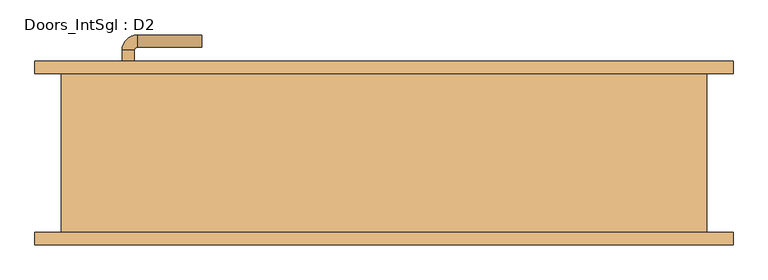
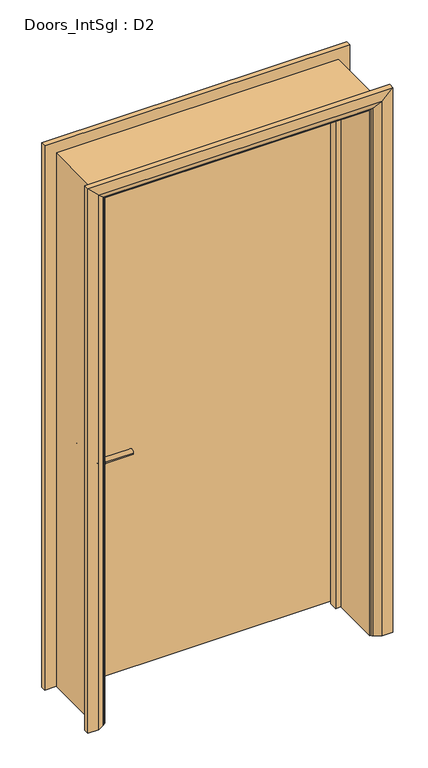
"""IFC4 building model written with IfcOpenShell, lengths in millimetres: door geometry, Doors_IntSgl : D2."""

from ifc_helpers import new_model, si_unit, point, frame, frame_2d, origin, place, context, project, spatial, polyline, circle_curve, ellipse_curve, trimmed, segment, composite_curve, outline, extrude, faceted_brep, source, transform, mapped, element, save
from ifc_brep_helpers import plane_surface, cylinder_surface, revolved_surface, advanced_brep


def doors_intsgl_d2_0f955423(model_context):
    return source(origin(), model_context, "Body", "SolidModel", [
        advanced_brep(
        [(-426.4, 83.54, 900.0), (-406.4, 83.54, 900.0), (-406.4, 53.54, 900.0), (-426.4, 53.54, 900.0), (-401.4, 48.54, 900.0), (-401.4, 28.54, 900.0), (-296.4, 28.54, 900.0), (-296.4, 48.54, 900.0)],
        [
            (0, 1, circle_curve(frame((-416.4, 83.54, 900.0), z_axis=(0.0, 1.0, 0.0), x_axis=(1.0, 0.0, 0.0)), 10.0)),
            (1, 0, circle_curve(frame((-416.4, 83.54, 900.0), z_axis=(0.0, 1.0, 0.0), x_axis=(1.0, 0.0, 0.0)), 10.0)),
            (1, 2),
            (2, 3, circle_curve(frame((-416.4, 53.54, 900.0), z_axis=(0.0, 1.0, 0.0), x_axis=(1.0, 0.0, 0.0)), 10.0)),
            (3, 0),
            (3, 2, circle_curve(frame((-416.4, 53.54, 900.0), z_axis=(0.0, 1.0, 0.0), x_axis=(1.0, 0.0, 0.0)), 10.0)),
            (4, 5, circle_curve(frame((-401.4, 38.54, 900.0), z_axis=(-1.0, 0.0, 0.0), x_axis=(0.0, 1.0, 0.0)), 10.0)),
            (5, 3, circle_curve(frame((-401.4, 53.54, 900.0), z_axis=(0.0, 0.0, -1.0), x_axis=(-1.0, 0.0, 0.0)), 25.0)),
            (2, 4, circle_curve(frame((-401.4, 53.54, 900.0), z_axis=(0.0, 0.0, 1.0), x_axis=(-1.0, 0.0, 0.0)), 5.0)),
            (5, 4, circle_curve(frame((-401.4, 38.54, 900.0), z_axis=(-1.0, 0.0, 0.0), x_axis=(0.0, 1.0, 0.0)), 10.0)),
            (6, 7, circle_curve(frame((-296.4, 38.54, 900.0), z_axis=(1.0, 0.0, 0.0), x_axis=(0.0, 1.0, 0.0)), 10.0)),
            (7, 6, circle_curve(frame((-296.4, 38.54, 900.0), z_axis=(1.0, 0.0, 0.0), x_axis=(0.0, 1.0, 0.0)), 10.0)),
            (4, 7),
            (6, 5),
        ],
        [
            plane_surface(frame((-416.4, 83.54, 900.0), z_axis=(0.0, 1.0, 0.0), x_axis=(0.0, 0.0, 1.0))),
            cylinder_surface(frame((-416.4, 83.54, 900.0), z_axis=(0.0, 1.0, 0.0), x_axis=(1.0, 0.0, 0.0)), 10.0),
            revolved_surface(trimmed(ellipse_curve(frame((-416.4, 53.54, 900.0), z_axis=(0.0, -1.0, 0.0), x_axis=(1.0, 0.0, 0.0)), 10.0, 10.0), [point((-426.4, 53.54, 900.0))], [point((-406.4, 53.54, 900.0))], True, "CARTESIAN"), (-401.4, 53.54, 900.0), (0.0, 0.0, -1.0)),
            revolved_surface(trimmed(ellipse_curve(frame((-416.4, 53.54, 900.0), z_axis=(0.0, -1.0, 0.0), x_axis=(1.0, 0.0, 0.0)), 10.0, 10.0), [point((-406.4, 53.54, 900.0))], [point((-426.4, 53.54, 900.0))], True, "CARTESIAN"), (-401.4, 53.54, 900.0), (0.0, 0.0, -1.0)),
            plane_surface(frame((-296.4, 38.54, 900.0), z_axis=(1.0, 0.0, 0.0), x_axis=(0.0, 0.0, 1.0))),
            cylinder_surface(frame((-401.4, 38.54, 900.0), z_axis=(-1.0, 0.0, 0.0), x_axis=(0.0, 1.0, 0.0)), 10.0),
        ],
        [
            (0, [[1, 2]]),
            (1, [[3, 4, 5, -2]]),
            (1, [[-5, 6, -3, -1]]),
            (2, [[7, 8, -4, 9]]),
            (3, [[10, -9, -6, -8]]),
            (4, [[11, 12]]),
            (5, [[13, -11, 14, -7]]),
            (5, [[-14, -12, -13, -10]]),
        ],
    ),
        extrude(outline(composite_curve([segment(trimmed(circle_curve(frame_2d((900.0, -418.9)), 30.0), [point((900.0, -448.9))], [point((900.0, -388.9))], False, "CARTESIAN"), True, "CONTINUOUS"), segment(trimmed(circle_curve(frame_2d((900.0, -418.9)), 30.0), [point((900.0, -388.9))], [point((900.0, -448.9))], False, "CARTESIAN"), True, "CONTINUOUS")], self_intersect=False)), frame((0.0, 83.54, 0.0), z_axis=(0.0, 1.0, 0.0), x_axis=(0.0, 0.0, 1.0)), (0.0, 0.0, 1.0), 8.0),
        advanced_brep(
        [(-426.4, 137.54, 900.0), (-406.4, 137.54, 900.0), (-426.4, 167.54, 900.0), (-406.4, 167.54, 900.0), (-401.4, 172.54, 900.0), (-401.4, 192.54, 900.0), (-296.4, 192.54, 900.0), (-296.4, 172.54, 900.0)],
        [
            (0, 1, circle_curve(frame((-416.4, 137.54, 900.0), z_axis=(0.0, -1.0, 0.0), x_axis=(1.0, 0.0, 0.0)), 10.0)),
            (1, 0, circle_curve(frame((-416.4, 137.54, 900.0), z_axis=(0.0, -1.0, 0.0), x_axis=(1.0, 0.0, 0.0)), 10.0)),
            (0, 2),
            (2, 3, circle_curve(frame((-416.4, 167.54, 900.0), z_axis=(0.0, -1.0, 0.0), x_axis=(1.0, 0.0, 0.0)), 10.0)),
            (3, 1),
            (3, 2, circle_curve(frame((-416.4, 167.54, 900.0), z_axis=(0.0, -1.0, 0.0), x_axis=(1.0, 0.0, 0.0)), 10.0)),
            (4, 3, circle_curve(frame((-401.4, 167.54, 900.0), z_axis=(0.0, 0.0, 1.0), x_axis=(-1.0, 0.0, 0.0)), 5.0)),
            (2, 5, circle_curve(frame((-401.4, 167.54, 900.0), z_axis=(0.0, 0.0, -1.0), x_axis=(-1.0, 0.0, 0.0)), 25.0)),
            (5, 4, circle_curve(frame((-401.4, 182.54, 900.0), z_axis=(-1.0, 0.0, 0.0), x_axis=(0.0, -1.0, 0.0)), 10.0)),
            (4, 5, circle_curve(frame((-401.4, 182.54, 900.0), z_axis=(-1.0, 0.0, 0.0), x_axis=(0.0, -1.0, 0.0)), 10.0)),
            (6, 7, circle_curve(frame((-296.4, 182.54, 900.0), z_axis=(1.0, 0.0, 0.0), x_axis=(0.0, -1.0, 0.0)), 10.0)),
            (7, 6, circle_curve(frame((-296.4, 182.54, 900.0), z_axis=(1.0, 0.0, 0.0), x_axis=(0.0, -1.0, 0.0)), 10.0)),
            (5, 6),
            (7, 4),
        ],
        [
            plane_surface(frame((-416.4, 137.54, 900.0), z_axis=(0.0, -1.0, 0.0), x_axis=(0.0, 0.0, 1.0))),
            cylinder_surface(frame((-416.4, 137.54, 900.0), z_axis=(0.0, -1.0, 0.0), x_axis=(1.0, 0.0, 0.0)), 10.0),
            revolved_surface(trimmed(ellipse_curve(frame((-416.4, 167.54, 900.0), z_axis=(0.0, -1.0, 0.0), x_axis=(1.0, 0.0, 0.0)), 10.0, 10.0), [point((-426.4, 167.54, 900.0))], [point((-406.4, 167.54, 900.0))], True, "CARTESIAN"), (-401.4, 167.54, 900.0), (0.0, 0.0, -1.0)),
            revolved_surface(trimmed(ellipse_curve(frame((-416.4, 167.54, 900.0), z_axis=(0.0, -1.0, 0.0), x_axis=(1.0, 0.0, 0.0)), 10.0, 10.0), [point((-406.4, 167.54, 900.0))], [point((-426.4, 167.54, 900.0))], True, "CARTESIAN"), (-401.4, 167.54, 900.0), (0.0, 0.0, -1.0)),
            plane_surface(frame((-296.4, 182.54, 900.0), z_axis=(1.0, 0.0, 0.0), x_axis=(0.0, 0.0, 1.0))),
            cylinder_surface(frame((-401.4, 182.54, 900.0), z_axis=(-1.0, 0.0, 0.0), x_axis=(0.0, -1.0, 0.0)), 10.0),
        ],
        [
            (0, [[1, 2]]),
            (1, [[-1, 3, 4, 5]]),
            (1, [[-2, -5, 6, -3]]),
            (2, [[7, -4, 8, 9]]),
            (3, [[-8, -6, -7, 10]]),
            (4, [[11, 12]]),
            (5, [[-9, 13, -12, 14]]),
            (5, [[-10, -14, -11, -13]]),
        ],
    ),
        extrude(outline(composite_curve([segment(trimmed(circle_curve(frame_2d((900.0, -418.9)), 30.0), [point((900.0, -448.9))], [point((900.0, -388.9))], False, "CARTESIAN"), True, "CONTINUOUS"), segment(trimmed(circle_curve(frame_2d((900.0, -418.9)), 30.0), [point((900.0, -388.9))], [point((900.0, -448.9))], False, "CARTESIAN"), True, "CONTINUOUS")], self_intersect=False)), frame((0.0, 129.54, 0.0), z_axis=(0.0, 1.0, 0.0), x_axis=(0.0, 0.0, 1.0)), (0.0, 0.0, 1.0), 8.0),
        extrude(outline(polyline([(491.4, 91.54), (-491.4, 91.54), (-491.4, 129.54), (491.4, 129.54), (491.4, 91.54)])), frame((0.0, 0.0, 8.0), z_axis=(0.0, 0.0, 1.0), x_axis=(1.0, 0.0, 0.0)), (0.0, 0.0, 1.0), 2060.0),
        advanced_brep(
        [(568.4, 149.54, 0.0), (568.4, 129.54, 0.0), (498.4, 129.54, 0.0), (502.4, 135.54, 0.0), (528.4, 149.54, 0.0), (568.4, 149.54, 2145.0), (568.4, 129.54, 2145.0), (-568.4, 129.54, 2145.0), (-568.4, 129.54, 0.0), (-498.4, 129.54, 0.0), (-498.4, 129.54, 2075.0), (498.4, 129.54, 2075.0), (502.4, 135.54, 2079.0), (528.4, 149.54, 2105.0), (-528.4, 149.54, 2105.0), (-528.4, 149.54, 0.0), (-568.4, 149.54, 0.0), (-568.4, 149.54, 2145.0), (-502.4, 135.54, 0.0), (-502.4, 135.54, 2079.0)],
        [
            (0, 1),
            (1, 2),
            (2, 3, circle_curve(frame((506.4, 128.54, 0.0), z_axis=(0.0, 0.0, -1.0), x_axis=(1.0, 0.0, 0.0)), 8.0622577)),
            (3, 4),
            (4, 0),
            (0, 5),
            (5, 6),
            (6, 1),
            (6, 7),
            (7, 8),
            (8, 9),
            (9, 10),
            (10, 11),
            (11, 2),
            (11, 12, ellipse_curve(frame((506.4, 128.54, 2083.0), z_axis=(0.7071067811865475, 0.0, -0.7071067811865475), x_axis=(-0.7071067811865474, 0.0, -0.7071067811865476)), 11.4017543, 8.0622577)),
            (12, 3),
            (12, 13),
            (13, 4),
            (13, 14),
            (14, 15),
            (15, 16),
            (16, 17),
            (17, 5),
            (7, 17),
            (16, 8),
            (15, 18),
            (18, 9, circle_curve(frame((-506.4, 128.54, 0.0), z_axis=(0.0, 0.0, -1.0), x_axis=(-1.0, 0.0, 0.0)), 8.0622577)),
            (19, 10, ellipse_curve(frame((-506.4, 128.54, 2083.0), z_axis=(-0.7071067811865475, 0.0, -0.7071067811865475), x_axis=(-0.7071067811865474, 0.0, 0.7071067811865476)), 11.4017543, 8.0622577)),
            (18, 19),
            (14, 19),
            (19, 12),
        ],
        [
            plane_surface(frame((498.4, 129.54, 0.0), z_axis=(0.0, 0.0, -1.0), x_axis=(0.0, -1.0, 0.0))),
            plane_surface(frame((568.4, 149.54, 0.0), z_axis=(1.0, 0.0, 0.0), x_axis=(0.0, 0.0, 1.0))),
            plane_surface(frame((568.4, 129.54, 0.0), z_axis=(0.0, -1.0, 0.0), x_axis=(0.0, 0.0, 1.0))),
            cylinder_surface(frame((506.4, 128.54, 0.0), z_axis=(0.0, 0.0, -1.0), x_axis=(1.0, 0.0, 0.0)), 8.0622577),
            plane_surface(frame((502.4, 135.54, 0.0), z_axis=(-0.4740998230350126, 0.880471099922178, 0.0), x_axis=(0.0, 0.0, 1.0))),
            plane_surface(frame((528.4, 149.54, 0.0), z_axis=(0.0, 1.0, 0.0), x_axis=(0.0, 0.0, 1.0))),
            plane_surface(frame((-568.4, 149.54, 2145.0), z_axis=(-1.0, 0.0, 0.0), x_axis=(0.0, 0.0, -1.0))),
            plane_surface(frame((-498.4, 129.54, 0.0), z_axis=(0.0, 0.0, -1.0), x_axis=(0.0, -1.0, 0.0))),
            cylinder_surface(frame((-506.4, 128.54, 2075.0), z_axis=(0.0, 0.0, 1.0), x_axis=(-1.0, 0.0, 0.0)), 8.0622577),
            plane_surface(frame((-502.4, 135.54, 2079.0), z_axis=(0.47409982303501824, 0.8804710999221749, 0.0), x_axis=(0.0, 0.0, -1.0))),
            plane_surface(frame((568.4, 149.54, 2145.0), z_axis=(0.0, 0.0, 1.0), x_axis=(-1.0, 0.0, 0.0))),
            cylinder_surface(frame((498.4, 128.54, 2083.0), z_axis=(1.0, 0.0, 0.0), x_axis=(0.0, 0.0, 1.0)), 8.0622577),
            plane_surface(frame((502.4, 135.54, 2079.0), z_axis=(0.0, 0.8804710999221764, -0.4740998230350154), x_axis=(-1.0, 0.0, 0.0))),
        ],
        [
            (0, [[1, 2, 3, 4, 5]]),
            (1, [[-1, 6, 7, 8]]),
            (2, [[-2, -8, 9, 10, 11, 12, 13, 14]]),
            (3, [[-3, -14, 15, 16]]),
            (4, [[-4, -16, 17, 18]]),
            (5, [[-5, -18, 19, 20, 21, 22, 23, -6]]),
            (6, [[24, -22, 25, -10]]),
            (7, [[-21, 26, 27, -11, -25]]),
            (8, [[28, -12, -27, 29]]),
            (9, [[30, -29, -26, -20]]),
            (10, [[-7, -23, -24, -9]]),
            (11, [[-15, -13, -28, 31]]),
            (12, [[-17, -31, -30, -19]]),
        ],
    ),
        extrude(outline(polyline([(0.0, -493.4), (0.0, -474.4), (2051.0, -474.4), (2051.0, 474.4), (0.0, 474.4), (0.0, 493.4), (2070.0, 493.4), (2070.0, -493.4), (0.0, -493.4)])), frame((0.0, 57.54, 0.0), z_axis=(0.0, 1.0, 0.0), x_axis=(0.0, 0.0, 1.0)), (0.0, 0.0, 1.0), 32.0),
        advanced_brep(
        [(-568.4, -149.54, 0.0), (-568.4, -129.54, 0.0), (-498.4, -129.54, 0.0), (-502.4, -135.54, 0.0), (-528.4, -149.54, 0.0), (-568.4, -149.54, 2145.0), (-568.4, -129.54, 2145.0), (-498.4, -129.54, 2075.0), (-502.4, -135.54, 2079.0), (-528.4, -149.54, 2105.0), (568.4, -149.54, 0.0), (528.4, -149.54, 0.0), (502.4, -135.54, 0.0), (498.4, -129.54, 0.0), (568.4, -129.54, 0.0), (568.4, -149.54, 2145.0), (528.4, -149.54, 2105.0), (502.4, -135.54, 2079.0), (498.4, -129.54, 2075.0), (568.4, -129.54, 2145.0)],
        [
            (0, 1),
            (1, 2),
            (2, 3, circle_curve(frame((-506.4, -128.54, 0.0), z_axis=(0.0, 0.0, -1.0), x_axis=(-1.0, 0.0, 0.0)), 8.0622577)),
            (3, 4),
            (4, 0),
            (0, 5),
            (5, 6),
            (6, 1),
            (6, 7),
            (7, 2),
            (7, 8, ellipse_curve(frame((-506.4, -128.54, 2083.0), z_axis=(-0.7071067811865475, 0.0, -0.7071067811865475), x_axis=(0.7071067811865474, 0.0, -0.7071067811865476)), 11.4017543, 8.0622577)),
            (8, 3),
            (8, 9),
            (9, 4),
            (9, 5),
            (10, 11),
            (11, 12),
            (12, 13, circle_curve(frame((506.4, -128.54, 0.0), z_axis=(0.0, 0.0, -1.0), x_axis=(1.0, 0.0, 0.0)), 8.0622577)),
            (13, 14),
            (14, 10),
            (15, 16),
            (16, 11),
            (10, 15),
            (16, 17),
            (17, 12),
            (17, 18, ellipse_curve(frame((506.4, -128.54, 2083.0), z_axis=(0.7071067811865475, 0.0, -0.7071067811865475), x_axis=(0.7071067811865474, 0.0, 0.7071067811865476)), 11.4017543, 8.0622577)),
            (18, 13),
            (18, 19),
            (19, 14),
            (19, 15),
            (5, 15),
            (19, 6),
            (18, 7),
            (17, 8),
            (16, 9),
        ],
        [
            plane_surface(frame((-498.4, -202.3410989, 0.0), z_axis=(0.0, 0.0, -1.0), x_axis=(1.0, 0.0, 0.0))),
            plane_surface(frame((-568.4, -149.54, 0.0), z_axis=(-1.0, 0.0, 0.0), x_axis=(0.0, 0.0, 1.0))),
            plane_surface(frame((-568.4, -129.54, 0.0), z_axis=(0.0, 1.0, 0.0), x_axis=(0.0, 0.0, 1.0))),
            cylinder_surface(frame((-506.4, -128.54, 0.0), z_axis=(0.0, 0.0, -1.0), x_axis=(-1.0, 0.0, 0.0)), 8.0622577),
            plane_surface(frame((-502.4, -135.54, 0.0), z_axis=(0.4740998230350183, -0.8804710999221749, 0.0), x_axis=(0.0, 0.0, 1.0))),
            plane_surface(frame((-528.4, -149.54, 0.0), z_axis=(0.0, -1.0, 0.0), x_axis=(0.0, 0.0, 1.0))),
            plane_surface(frame((498.4, -202.3410989, 0.0), z_axis=(0.0, 0.0, -1.0), x_axis=(-1.0, 0.0, 0.0))),
            plane_surface(frame((528.4, -149.54, 2105.0), z_axis=(0.0, -1.0, 0.0), x_axis=(0.0, 0.0, -1.0))),
            plane_surface(frame((502.4, -135.54, 2079.0), z_axis=(-0.4740998230350183, -0.8804710999221749, 0.0), x_axis=(0.0, 0.0, -1.0))),
            cylinder_surface(frame((506.4, -128.54, 2075.0), z_axis=(0.0, 0.0, 1.0), x_axis=(1.0, 0.0, 0.0)), 8.0622577),
            plane_surface(frame((568.4, -129.54, 2145.0), z_axis=(0.0, 1.0, 0.0), x_axis=(0.0, 0.0, -1.0))),
            plane_surface(frame((568.4, -149.54, 2145.0), z_axis=(1.0, 0.0, 0.0), x_axis=(0.0, 0.0, -1.0))),
            plane_surface(frame((-568.4, -149.54, 2145.0), z_axis=(0.0, 0.0, 1.0), x_axis=(1.0, 0.0, 0.0))),
            plane_surface(frame((-568.4, -129.54, 2145.0), z_axis=(0.0, 1.0, 0.0), x_axis=(1.0, 0.0, 0.0))),
            cylinder_surface(frame((-498.4, -128.54, 2083.0), z_axis=(-1.0, 0.0, 0.0), x_axis=(0.0, 0.0, 1.0)), 8.0622577),
            plane_surface(frame((-502.4, -135.54, 2079.0), z_axis=(0.0, -0.8804710999221749, -0.4740998230350183), x_axis=(1.0, 0.0, 0.0))),
            plane_surface(frame((-528.4, -149.54, 2105.0), z_axis=(0.0, -1.0, 0.0), x_axis=(1.0, 0.0, 0.0))),
        ],
        [
            (0, [[1, 2, 3, 4, 5]]),
            (1, [[-1, 6, 7, 8]]),
            (2, [[-2, -8, 9, 10]]),
            (3, [[-3, -10, 11, 12]]),
            (4, [[-4, -12, 13, 14]]),
            (5, [[-5, -14, 15, -6]]),
            (6, [[16, 17, 18, 19, 20]]),
            (7, [[21, 22, -16, 23]]),
            (8, [[24, 25, -17, -22]]),
            (9, [[26, 27, -18, -25]]),
            (10, [[28, 29, -19, -27]]),
            (11, [[30, -23, -20, -29]]),
            (12, [[-7, 31, -30, 32]]),
            (13, [[-9, -32, -28, 33]]),
            (14, [[-11, -33, -26, 34]]),
            (15, [[-13, -34, -24, 35]]),
            (16, [[-15, -35, -21, -31]]),
        ],
    ),
        faceted_brep([(-493.4, 129.54, 0.0), (-493.4, -129.54, 0.0), (-525.4, -129.54, 0.0), (-525.4, 129.54, 0.0), (-493.4, 129.54, 2070.0), (-493.4, -129.54, 2070.0), (-525.4, -129.54, 2102.0), (-525.4, 129.54, 2102.0), (493.4, 129.54, 0.0), (525.4, 129.54, 0.0), (525.4, -129.54, 0.0), (493.4, -129.54, 0.0), (493.4, 129.54, 2070.0), (525.4, 129.54, 2102.0), (525.4, -129.54, 2102.0), (493.4, -129.54, 2070.0)], [[[0, 1, 2, 3]], [[1, 0, 4, 5]], [[2, 1, 5, 6]], [[3, 2, 6, 7]], [[0, 3, 7, 4]], [[8, 9, 10, 11]], [[12, 13, 9, 8]], [[13, 14, 10, 9]], [[14, 15, 11, 10]], [[15, 12, 8, 11]], [[5, 4, 12, 15]], [[6, 5, 15, 14]], [[7, 6, 14, 13]], [[4, 7, 13, 12]]]),
    ])


if __name__ == "__main__":
    model = new_model("IFC4")
    model_context = context("Model", 3, world=origin())
    ifc_project = project(units=[si_unit("LENGTHUNIT", "METRE", prefix="MILLI")], contexts=[model_context])
    site = spatial("IfcSite", under=ifc_project)
    building = spatial("IfcBuilding", under=site)
    placement = place(None, origin())
    doors_intsgl_d2_shape = doors_intsgl_d2_0f955423(model_context)
    element("IfcDoor", 1, ObjectType="Doors_IntSgl : D2", at=placement, inside=building, context=model_context, shape_type="MappedRepresentation", body=[
        mapped(doors_intsgl_d2_shape, transform((0.0, 0.0, 0.0), x_axis=(1.0, 0.0, 0.0), y_axis=(0.0, 1.0, 0.0), z_axis=(0.0, 0.0, 1.0))),
    ])
    save(model, "model.ifc")

# Revit data of these elements
# Type "Doors_IntSgl : D2"
#   Type Mark = "47"
#   Type Comments = "Internal Single"
#   Operation = "SingleSwingRight"
#   Manufacturer = "Revit"
#   Keynote = "L20"
#   Description = "Internal Single Door"
#   Analytic Construction = "Metal"
#   UnderCut = 8 mm
#   Tolerance = 2 mm
#   Thickness = 38 mm
#   Thermal Resistance (R) = 0.270117 (m²·K)/W
#   Structural Tolerance = 8 mm
#   StopDepth = 32 mm
#   Stop Thickness = 19 mm
#   Rough Width = 1066.8 mm
#   Rough Height = 2110 mm
#   Height to Top Lock Rail = 1000 mm
#   Heat Transfer Coefficient (U) = 3.7021 W/(m²·K)
#   Handle Z Distance = 900 mm
#   Handle X Distance = 75 mm
#   Frame Thickness = 32 mm
#   Door Panel Width = 982.8 mm
#   Door Panel Thickness = 38 mm
#   Door Panel Offset = 0 mm
#   Height = 2110 mm
#   Width = 1066.8 mm
#   Door Panel Height = 2060 mm
#   Architrave Setback = 5 mm
#   Vis - Ironmongery = yes
#   Material Ironmongery = Door - Handle
#   Material Frame = Door - Frame/Mullion (1)
#   Material Door = Door - Panel
#   Material Architrave = Door - Architrave
#   Visual Light Transmittance = 0
#   Solar Heat Gain Coefficient = 0
#   Function = (empty or 0)
#   Wall Closure = (empty or 0)
# Element 1 (IfcDoor, "Doors_IntSgl : D2")
#   Materials on its faces: "Door - Architrave", "Door - Handle", "Door - Frame/Mullion (1)", "Door - Panel"
# Materials
#   "Door - Handle": colour RGB 0 0 0, transparency 0, Keynote = "P21", Cost = 0
#   "Door - Frame/Mullion (1)": class "Wood", colour RGB 212 179 113, transparency 0, Keynote = "L20", Cost = 0
#   "Door - Panel": class "Wood", colour RGB 210 159 95, transparency 0, Keynote = "L20", Cost = 0
#   "Door - Architrave": class "Wood", colour RGB 154 90 5, transparency 0, Keynote = "P20", Cost = 0
